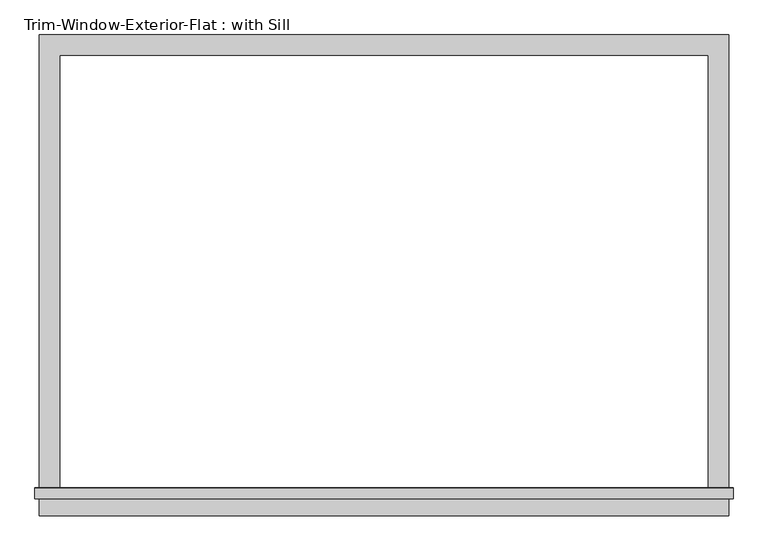
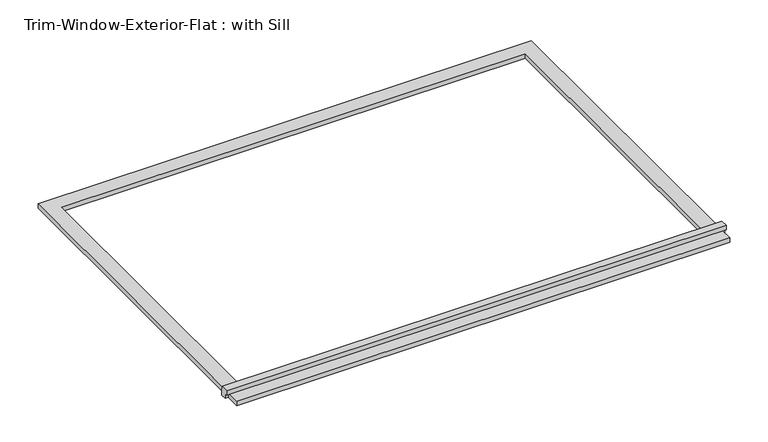
"""IFC4 building model written with IfcOpenShell, lengths in millimetres: proxy geometry, Trim-Window-Exterior-Flat : with Sill."""

from ifc_helpers import new_model, si_unit, frame, origin, origin_with_axes, place, context, project, spatial, polyline, outline, extrude, source, transform, mapped, element, save


def trim_window_exterior_flat_with_sill_02d88a07(model_context):
    return source(origin(), model_context, "Body", "SweptSolid", [
        extrude(outline(polyline([(971.55, -1241.3823709), (971.55, -1298.5323709), (-971.55, -1298.5323709), (-971.55, -1241.3823709), (971.55, -1241.3823709)])), origin_with_axes(), (0.0, 0.0, 1.0), 19.05),
        extrude(outline(polyline([(-1250.95, 38.1), (-1221.6580645, 38.1), (-1219.2, 19.05), (-1219.2, 0.0), (-1241.3823709, 0.0), (-1241.3823709, 19.05), (-1250.95, 19.05), (-1250.95, 38.1)])), frame((-984.25, 0.0, 0.0), z_axis=(1.0, 0.0, 0.0), x_axis=(0.0, 1.0, 0.0)), (0.0, 0.0, 1.0), 1968.5),
        extrude(outline(polyline([(-971.55, 57.15), (971.55, 57.15), (971.55, -1219.2), (914.4, -1219.2), (914.4, 0.0), (-914.4, 0.0), (-914.4, -1219.2), (-971.55, -1219.2), (-971.55, 57.15)])), origin_with_axes(), (0.0, 0.0, 1.0), 19.05),
    ])


if __name__ == "__main__":
    model = new_model("IFC4")
    model_context = context("Model", 3, world=origin())
    ifc_project = project(units=[si_unit("LENGTHUNIT", "METRE", prefix="MILLI")], contexts=[model_context])
    site = spatial("IfcSite", under=ifc_project)
    building = spatial("IfcBuilding", under=site)
    placement = place(None, origin())
    trim_window_exterior_flat_with_sill_shape = trim_window_exterior_flat_with_sill_02d88a07(model_context)
    element("IfcBuildingElementProxy", 1, Name="Trim-Window-Exterior-Flat : with Sill", ObjectType="Trim-Window-Exterior-Flat : with Sill", at=placement, inside=building, context=model_context, shape_type="MappedRepresentation", body=[
        mapped(trim_window_exterior_flat_with_sill_shape, transform((0.0, 0.0, 0.0), x_axis=(1.0, 0.0, 0.0), y_axis=(0.0, 1.0, 0.0), z_axis=(0.0, 0.0, 1.0))),
    ])
    save(model, "model.ifc")

# Revit data of these elements
# Type "Trim-Window-Exterior-Flat : with Sill"
#   Trim Width = 0' - 2 1/4"
#   Trim Thickness_Picture Frame = 0' - 1 1/4"
#   Trim Thickness_with Sill = 0' - 0 3/4"
#   Sill Thickness = 0' - 1 1/4"
#   Opening Width [instance default] = 2' - 0"
#   Opening Height [instance default] = 3' - 0"
#   Default Elevation = 4' - 0"
#   Sill = yes
#   Picture Frame = no
#   Trim Material [instance default] = none
# Element 1 (IfcBuildingElementProxy, "Trim-Window-Exterior-Flat : with Sill")
#   Opening Width = 6' - 0"
#   Opening Height = 4' - 0"
#   Trim Material = Clad - White
#   Materials on its faces: "Clad - White"
# Materials
#   "Clad - White": class "Wood", colour RGB 242 242 238, transparency 0, Cost = 0
